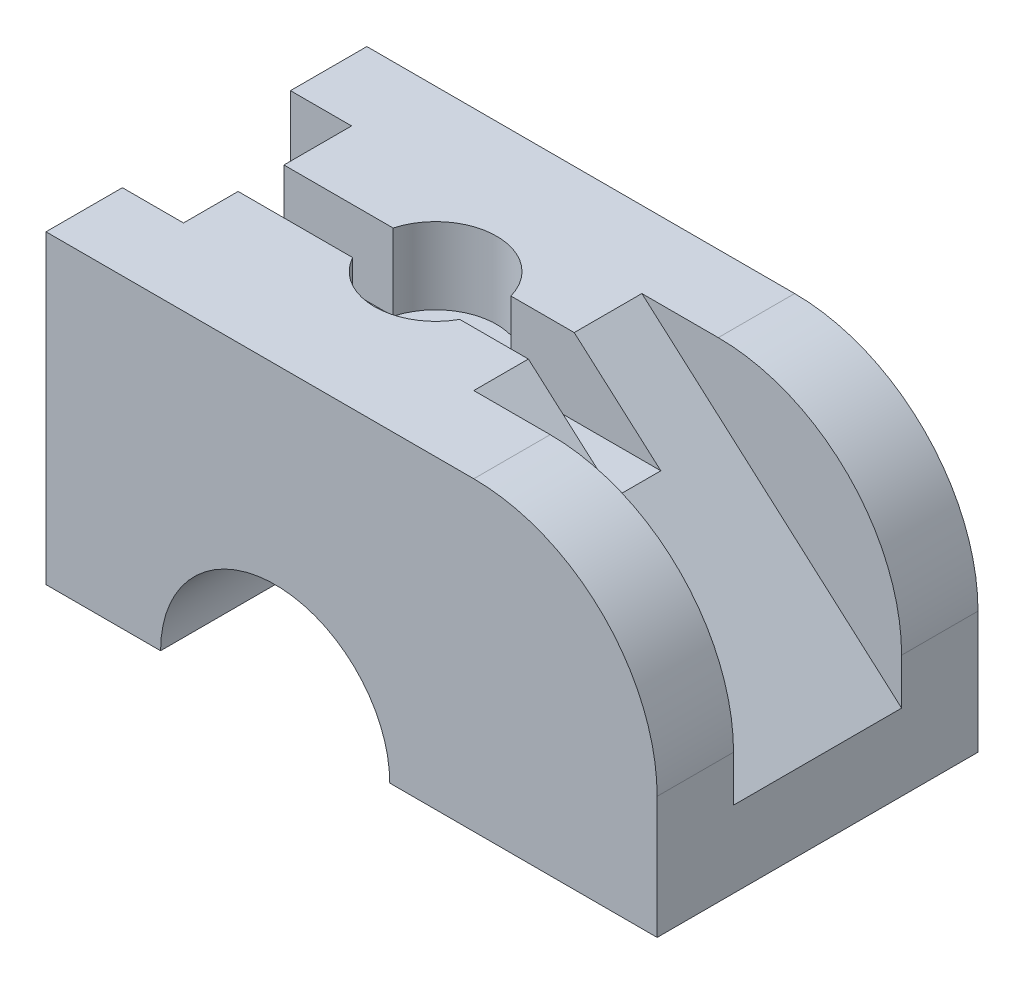
ISO-10303-21;
HEADER;
FILE_DESCRIPTION(('STEP AP214'),'2;1');
FILE_NAME('part.step','',(''),(''),'','','');
FILE_SCHEMA(('AUTOMOTIVE_DESIGN { 1 0 10303 214 1 1 1 1 }'));
ENDSEC;
DATA;
#1=APPLICATION_CONTEXT('core data for automotive mechanical design processes');
#2=APPLICATION_PROTOCOL_DEFINITION('international standard','automotive_design',2000,#1);
#3=PRODUCT_CONTEXT('',#1,'mechanical');
#4=PRODUCT('Part','Part','',(#3));
#5=PRODUCT_RELATED_PRODUCT_CATEGORY('part','',(#4));
#6=PRODUCT_DEFINITION_FORMATION('','',#4);
#7=PRODUCT_DEFINITION_CONTEXT('part definition',#1,'design');
#8=PRODUCT_DEFINITION('design','',#6,#7);
#9=PRODUCT_DEFINITION_SHAPE('','',#8);
#10=(LENGTH_UNIT() NAMED_UNIT(*) SI_UNIT(.MILLI.,.METRE.));
#11=(NAMED_UNIT(*) PLANE_ANGLE_UNIT() SI_UNIT($,.RADIAN.));
#12=(NAMED_UNIT(*) SI_UNIT($,.STERADIAN.) SOLID_ANGLE_UNIT());
#13=UNCERTAINTY_MEASURE_WITH_UNIT(LENGTH_MEASURE(1.E-05),#10,'distance_accuracy_value','');
#14=(GEOMETRIC_REPRESENTATION_CONTEXT(3) GLOBAL_UNCERTAINTY_ASSIGNED_CONTEXT((#13)) GLOBAL_UNIT_ASSIGNED_CONTEXT((#10,
#11,#12)) REPRESENTATION_CONTEXT('',''));
#15=CARTESIAN_POINT('',(0.,0.,0.));
#16=DIRECTION('',(0.,0.,1.));
#17=DIRECTION('',(1.,0.,0.));
#18=AXIS2_PLACEMENT_3D('',#15,#16,#17);
#19=CARTESIAN_POINT('',(-40.,0.,-42.));
#20=DIRECTION('',(-1.,0.,0.));
#21=DIRECTION('',(0.,0.,1.));
#22=AXIS2_PLACEMENT_3D('',#19,#20,#21);
#23=PLANE('',#22);
#24=DIRECTION('',(0.,1.,0.));
#25=VECTOR('',#24,1.);
#26=CARTESIAN_POINT('',(-40.,-2.,-32.));
#27=LINE('',#26,#25);
#28=CARTESIAN_POINT('',(-40.,0.,-32.));
#29=VERTEX_POINT('',#28);
#30=CARTESIAN_POINT('',(-40.,40.,-32.));
#31=VERTEX_POINT('',#30);
#32=EDGE_CURVE('E392',#29,#31,#27,.T.);
#33=ORIENTED_EDGE('',*,*,#32,.T.);
#34=DIRECTION('',(0.,0.,1.));
#35=VECTOR('',#34,1.);
#36=CARTESIAN_POINT('',(-40.,40.,-42.));
#37=LINE('',#36,#35);
#38=CARTESIAN_POINT('',(-40.,40.,-42.));
#39=VERTEX_POINT('',#38);
#40=EDGE_CURVE('E226',#39,#31,#37,.T.);
#41=ORIENTED_EDGE('',*,*,#40,.F.);
#42=DIRECTION('',(0.,-1.,0.));
#43=VECTOR('',#42,1.);
#44=CARTESIAN_POINT('',(-40.,0.,-42.));
#45=LINE('',#44,#43);
#46=CARTESIAN_POINT('',(-40.,0.,-42.));
#47=VERTEX_POINT('',#46);
#48=EDGE_CURVE('E335',#39,#47,#45,.T.);
#49=ORIENTED_EDGE('',*,*,#48,.T.);
#50=DIRECTION('',(0.,0.,1.));
#51=VECTOR('',#50,1.);
#52=CARTESIAN_POINT('',(-40.,0.,-42.));
#53=LINE('',#52,#51);
#54=EDGE_CURVE('E238',#47,#29,#53,.T.);
#55=ORIENTED_EDGE('',*,*,#54,.T.);
#56=EDGE_LOOP('',(#33,#41,#49,#55));
#57=FACE_BOUND('',#56,.T.);
#58=ADVANCED_FACE('F50',(#57),#23,.T.);
#59=CARTESIAN_POINT('',(-40.,0.,-42.));
#60=DIRECTION('',(0.,-1.,0.));
#61=DIRECTION('',(0.,0.,-1.));
#62=AXIS2_PLACEMENT_3D('',#59,#60,#61);
#63=PLANE('',#62);
#64=DIRECTION('',(0.,0.,1.));
#65=VECTOR('',#64,1.);
#66=CARTESIAN_POINT('',(5.,0.,-42.));
#67=LINE('',#66,#65);
#68=CARTESIAN_POINT('',(5.,0.,-42.));
#69=VERTEX_POINT('',#68);
#70=CARTESIAN_POINT('',(5.,0.,0.));
#71=VERTEX_POINT('',#70);
#72=EDGE_CURVE('E69',#69,#71,#67,.T.);
#73=ORIENTED_EDGE('',*,*,#72,.F.);
#74=DIRECTION('',(1.,0.,0.));
#75=VECTOR('',#74,1.);
#76=CARTESIAN_POINT('',(-40.,0.,-42.));
#77=LINE('',#76,#75);
#78=CARTESIAN_POINT('',(40.,0.,-42.));
#79=VERTEX_POINT('',#78);
#80=EDGE_CURVE('E323',#69,#79,#77,.T.);
#81=ORIENTED_EDGE('',*,*,#80,.T.);
#82=DIRECTION('',(0.,0.,1.));
#83=VECTOR('',#82,1.);
#84=CARTESIAN_POINT('',(40.,0.,-42.));
#85=LINE('',#84,#83);
#86=CARTESIAN_POINT('',(40.,0.,0.));
#87=VERTEX_POINT('',#86);
#88=EDGE_CURVE('E242',#79,#87,#85,.T.);
#89=ORIENTED_EDGE('',*,*,#88,.T.);
#90=DIRECTION('',(1.,0.,0.));
#91=VECTOR('',#90,1.);
#92=CARTESIAN_POINT('',(-40.,0.,0.));
#93=LINE('',#92,#91);
#94=EDGE_CURVE('E295',#71,#87,#93,.T.);
#95=ORIENTED_EDGE('',*,*,#94,.F.);
#96=EDGE_LOOP('',(#73,#81,#89,#95));
#97=FACE_BOUND('',#96,.T.);
#98=ADVANCED_FACE('F321',(#97),#63,.T.);
#99=CARTESIAN_POINT('',(6.,40.,-42.));
#100=DIRECTION('',(-0.661621637086846,-0.749837855365093,0.));
#101=DIRECTION('',(0.749837855365093,-0.661621637086846,0.));
#102=AXIS2_PLACEMENT_3D('',#99,#100,#101);
#103=PLANE('',#102);
#104=DIRECTION('',(0.,0.,1.));
#105=VECTOR('',#104,1.);
#106=CARTESIAN_POINT('',(40.,10.,-42.));
#107=LINE('',#106,#105);
#108=CARTESIAN_POINT('',(40.,10.,-32.));
#109=VERTEX_POINT('',#108);
#110=CARTESIAN_POINT('',(40.,10.,-10.));
#111=VERTEX_POINT('',#110);
#112=EDGE_CURVE('E281',#109,#111,#107,.T.);
#113=ORIENTED_EDGE('',*,*,#112,.F.);
#114=DIRECTION('',(-0.749837855365093,0.661621637086846,0.));
#115=VECTOR('',#114,1.);
#116=CARTESIAN_POINT('',(6.,40.,-32.));
#117=LINE('',#116,#115);
#118=CARTESIAN_POINT('',(6.,40.,-32.));
#119=VERTEX_POINT('',#118);
#120=EDGE_CURVE('E282',#109,#119,#117,.T.);
#121=ORIENTED_EDGE('',*,*,#120,.T.);
#122=DIRECTION('',(0.,0.,1.));
#123=VECTOR('',#122,1.);
#124=CARTESIAN_POINT('',(6.,40.,-42.));
#125=LINE('',#124,#123);
#126=CARTESIAN_POINT('',(6.,40.,-23.147915887961));
#127=VERTEX_POINT('',#126);
#128=EDGE_CURVE('E374',#119,#127,#125,.T.);
#129=ORIENTED_EDGE('',*,*,#128,.T.);
#130=DIRECTION('',(0.749837855365093,-0.661621637086846,0.));
#131=VECTOR('',#130,1.);
#132=CARTESIAN_POINT('',(6.,40.,-23.147915887961));
#133=LINE('',#132,#131);
#134=CARTESIAN_POINT('',(17.3333333333333,30.,-23.147915887961));
#135=VERTEX_POINT('',#134);
#136=EDGE_CURVE('E239',#127,#135,#133,.T.);
#137=ORIENTED_EDGE('',*,*,#136,.T.);
#138=DIRECTION('',(0.,0.,1.));
#139=VECTOR('',#138,1.);
#140=CARTESIAN_POINT('',(17.3333333333333,30.,-42.));
#141=LINE('',#140,#139);
#142=CARTESIAN_POINT('',(17.3333333333333,30.,-17.147915887961));
#143=VERTEX_POINT('',#142);
#144=EDGE_CURVE('E243',#135,#143,#141,.T.);
#145=ORIENTED_EDGE('',*,*,#144,.T.);
#146=DIRECTION('',(-0.749837855365093,0.661621637086846,0.));
#147=VECTOR('',#146,1.);
#148=CARTESIAN_POINT('',(5.99999999999999,40.,-17.147915887961));
#149=LINE('',#148,#147);
#150=CARTESIAN_POINT('',(6.,40.,-17.147915887961));
#151=VERTEX_POINT('',#150);
#152=EDGE_CURVE('E250',#143,#151,#149,.T.);
#153=ORIENTED_EDGE('',*,*,#152,.T.);
#154=CARTESIAN_POINT('',(6.,40.,-10.));
#155=VERTEX_POINT('',#154);
#156=EDGE_CURVE('E380',#151,#155,#125,.T.);
#157=ORIENTED_EDGE('',*,*,#156,.T.);
#158=DIRECTION('',(-0.749837855365093,0.661621637086846,0.));
#159=VECTOR('',#158,1.);
#160=CARTESIAN_POINT('',(6.,40.,-10.));
#161=LINE('',#160,#159);
#162=EDGE_CURVE('E248',#111,#155,#161,.T.);
#163=ORIENTED_EDGE('',*,*,#162,.F.);
#164=EDGE_LOOP('',(#113,#121,#129,#137,#145,#153,#157,#163));
#165=FACE_BOUND('',#164,.T.);
#166=ADVANCED_FACE('F430',(#165),#103,.F.);
#167=CARTESIAN_POINT('',(-40.,40.,-42.));
#168=DIRECTION('',(0.,1.,0.));
#169=DIRECTION('',(0.,0.,1.));
#170=AXIS2_PLACEMENT_3D('',#167,#168,#169);
#171=PLANE('',#170);
#172=DIRECTION('',(-1.,0.,0.));
#173=VECTOR('',#172,1.);
#174=CARTESIAN_POINT('',(-40.,40.,-32.));
#175=LINE('',#174,#173);
#176=CARTESIAN_POINT('',(-32.,40.,-32.));
#177=VERTEX_POINT('',#176);
#178=EDGE_CURVE('E215',#177,#31,#175,.T.);
#179=ORIENTED_EDGE('',*,*,#178,.F.);
#180=DIRECTION('',(0.,0.,-1.));
#181=VECTOR('',#180,1.);
#182=CARTESIAN_POINT('',(-32.,40.,-32.));
#183=LINE('',#182,#181);
#184=CARTESIAN_POINT('',(-32.,40.,-23.147915887961));
#185=VERTEX_POINT('',#184);
#186=EDGE_CURVE('E225',#185,#177,#183,.T.);
#187=ORIENTED_EDGE('',*,*,#186,.F.);
#188=DIRECTION('',(-1.,0.,0.));
#189=VECTOR('',#188,1.);
#190=CARTESIAN_POINT('',(-40.,40.,-23.147915887961));
#191=LINE('',#190,#189);
#192=CARTESIAN_POINT('',(-17.7062609181266,40.,-23.147915887961));
#193=VERTEX_POINT('',#192);
#194=EDGE_CURVE('E358',#193,#185,#191,.T.);
#195=ORIENTED_EDGE('',*,*,#194,.F.);
#196=CARTESIAN_POINT('',(-10.,40.,-21.));
#197=DIRECTION('',(0.,1.,0.));
#198=DIRECTION('',(0.,0.,1.));
#199=AXIS2_PLACEMENT_3D('',#196,#197,#198);
#200=CIRCLE('',#199,8.);
#201=CARTESIAN_POINT('',(-2.29373908187345,40.,-23.147915887961));
#202=VERTEX_POINT('',#201);
#203=EDGE_CURVE('E360',#202,#193,#200,.T.);
#204=ORIENTED_EDGE('',*,*,#203,.F.);
#205=DIRECTION('',(-1.,0.,0.));
#206=VECTOR('',#205,1.);
#207=CARTESIAN_POINT('',(-2.29373908187345,40.,-23.147915887961));
#208=LINE('',#207,#206);
#209=EDGE_CURVE('E343',#127,#202,#208,.T.);
#210=ORIENTED_EDGE('',*,*,#209,.F.);
#211=ORIENTED_EDGE('',*,*,#128,.F.);
#212=DIRECTION('',(1.,0.,0.));
#213=VECTOR('',#212,1.);
#214=CARTESIAN_POINT('',(-40.,40.,-32.));
#215=LINE('',#214,#213);
#216=CARTESIAN_POINT('',(16.,40.,-32.));
#217=VERTEX_POINT('',#216);
#218=EDGE_CURVE('E322',#119,#217,#215,.T.);
#219=ORIENTED_EDGE('',*,*,#218,.T.);
#220=DIRECTION('',(0.,0.,-1.));
#221=VECTOR('',#220,1.);
#222=CARTESIAN_POINT('',(16.,40.,-42.));
#223=LINE('',#222,#221);
#224=CARTESIAN_POINT('',(16.,40.,-42.));
#225=VERTEX_POINT('',#224);
#226=EDGE_CURVE('E255',#217,#225,#223,.T.);
#227=ORIENTED_EDGE('',*,*,#226,.T.);
#228=DIRECTION('',(-1.,0.,0.));
#229=VECTOR('',#228,1.);
#230=CARTESIAN_POINT('',(6.,40.,-42.));
#231=LINE('',#230,#229);
#232=EDGE_CURVE('E305',#225,#39,#231,.T.);
#233=ORIENTED_EDGE('',*,*,#232,.T.);
#234=ORIENTED_EDGE('',*,*,#40,.T.);
#235=EDGE_LOOP('',(#179,#187,#195,#204,#210,#211,#219,#227,#233,#234));
#236=FACE_BOUND('',#235,.T.);
#237=ADVANCED_FACE('F407',(#236),#171,.T.);
#238=CARTESIAN_POINT('',(40.,15.9999999999998,-42.));
#239=DIRECTION('',(1.,0.,0.));
#240=DIRECTION('',(0.,0.,-1.));
#241=AXIS2_PLACEMENT_3D('',#238,#239,#240);
#242=PLANE('',#241);
#243=DIRECTION('',(0.,1.,0.));
#244=VECTOR('',#243,1.);
#245=CARTESIAN_POINT('',(40.,0.,-42.));
#246=LINE('',#245,#244);
#247=CARTESIAN_POINT('',(40.,16.,-42.));
#248=VERTEX_POINT('',#247);
#249=EDGE_CURVE('E230',#79,#248,#246,.T.);
#250=ORIENTED_EDGE('',*,*,#249,.T.);
#251=DIRECTION('',(0.,0.,-1.));
#252=VECTOR('',#251,1.);
#253=CARTESIAN_POINT('',(40.,16.,-42.));
#254=LINE('',#253,#252);
#255=CARTESIAN_POINT('',(40.,16.,-32.));
#256=VERTEX_POINT('',#255);
#257=EDGE_CURVE('E257',#248,#256,#254,.F.);
#258=ORIENTED_EDGE('',*,*,#257,.T.);
#259=DIRECTION('',(0.,-1.,0.));
#260=VECTOR('',#259,1.);
#261=CARTESIAN_POINT('',(40.,40.,-32.));
#262=LINE('',#261,#260);
#263=EDGE_CURVE('E385',#256,#109,#262,.T.);
#264=ORIENTED_EDGE('',*,*,#263,.T.);
#265=ORIENTED_EDGE('',*,*,#112,.T.);
#266=DIRECTION('',(0.,1.,0.));
#267=VECTOR('',#266,1.);
#268=CARTESIAN_POINT('',(40.,40.,-10.));
#269=LINE('',#268,#267);
#270=CARTESIAN_POINT('',(40.,16.,-10.));
#271=VERTEX_POINT('',#270);
#272=EDGE_CURVE('E271',#111,#271,#269,.T.);
#273=ORIENTED_EDGE('',*,*,#272,.T.);
#274=DIRECTION('',(0.,0.,1.));
#275=VECTOR('',#274,1.);
#276=CARTESIAN_POINT('',(40.,16.,-42.));
#277=LINE('',#276,#275);
#278=CARTESIAN_POINT('',(40.,16.,0.));
#279=VERTEX_POINT('',#278);
#280=EDGE_CURVE('E256',#271,#279,#277,.T.);
#281=ORIENTED_EDGE('',*,*,#280,.T.);
#282=DIRECTION('',(0.,1.,0.));
#283=VECTOR('',#282,1.);
#284=CARTESIAN_POINT('',(40.,15.9999999999998,0.));
#285=LINE('',#284,#283);
#286=EDGE_CURVE('E293',#87,#279,#285,.T.);
#287=ORIENTED_EDGE('',*,*,#286,.F.);
#288=ORIENTED_EDGE('',*,*,#88,.F.);
#289=EDGE_LOOP('',(#250,#258,#264,#265,#273,#281,#287,#288));
#290=FACE_BOUND('',#289,.T.);
#291=ADVANCED_FACE('F278',(#290),#242,.T.);
#292=DIRECTION('',(1.,0.,0.));
#293=VECTOR('',#292,1.);
#294=CARTESIAN_POINT('',(-40.,0.,-32.));
#295=LINE('',#294,#293);
#296=CARTESIAN_POINT('',(-32.,0.,-32.));
#297=VERTEX_POINT('',#296);
#298=EDGE_CURVE('E318',#29,#297,#295,.T.);
#299=ORIENTED_EDGE('',*,*,#298,.F.);
#300=ORIENTED_EDGE('',*,*,#54,.F.);
#301=CARTESIAN_POINT('',(-25.,0.,-42.));
#302=VERTEX_POINT('',#301);
#303=EDGE_CURVE('E234',#47,#302,#77,.T.);
#304=ORIENTED_EDGE('',*,*,#303,.T.);
#305=DIRECTION('',(0.,0.,1.));
#306=VECTOR('',#305,1.);
#307=CARTESIAN_POINT('',(-25.,0.,-42.));
#308=LINE('',#307,#306);
#309=CARTESIAN_POINT('',(-25.,0.,0.));
#310=VERTEX_POINT('',#309);
#311=EDGE_CURVE('E320',#302,#310,#308,.T.);
#312=ORIENTED_EDGE('',*,*,#311,.T.);
#313=CARTESIAN_POINT('',(-40.,0.,0.));
#314=VERTEX_POINT('',#313);
#315=EDGE_CURVE('E297',#314,#310,#93,.T.);
#316=ORIENTED_EDGE('',*,*,#315,.F.);
#317=CARTESIAN_POINT('',(-40.,0.,-10.));
#318=VERTEX_POINT('',#317);
#319=EDGE_CURVE('E235',#318,#314,#53,.T.);
#320=ORIENTED_EDGE('',*,*,#319,.F.);
#321=DIRECTION('',(-1.,0.,0.));
#322=VECTOR('',#321,1.);
#323=CARTESIAN_POINT('',(-40.,0.,-10.));
#324=LINE('',#323,#322);
#325=CARTESIAN_POINT('',(-32.,0.,-10.));
#326=VERTEX_POINT('',#325);
#327=EDGE_CURVE('E206',#326,#318,#324,.T.);
#328=ORIENTED_EDGE('',*,*,#327,.F.);
#329=DIRECTION('',(0.,0.,1.));
#330=VECTOR('',#329,1.);
#331=CARTESIAN_POINT('',(-32.,0.,-42.));
#332=LINE('',#331,#330);
#333=EDGE_CURVE('E387',#297,#326,#332,.T.);
#334=ORIENTED_EDGE('',*,*,#333,.F.);
#335=EDGE_LOOP('',(#299,#300,#304,#312,#316,#320,#328,#334));
#336=FACE_BOUND('',#335,.T.);
#337=ADVANCED_FACE('F314',(#336),#63,.T.);
#338=DIRECTION('',(0.,1.,0.));
#339=VECTOR('',#338,1.);
#340=CARTESIAN_POINT('',(-40.,-2.,-10.));
#341=LINE('',#340,#339);
#342=CARTESIAN_POINT('',(-40.,40.,-10.));
#343=VERTEX_POINT('',#342);
#344=EDGE_CURVE('E201',#318,#343,#341,.T.);
#345=ORIENTED_EDGE('',*,*,#344,.F.);
#346=ORIENTED_EDGE('',*,*,#319,.T.);
#347=DIRECTION('',(0.,-1.,0.));
#348=VECTOR('',#347,1.);
#349=CARTESIAN_POINT('',(-40.,0.,0.));
#350=LINE('',#349,#348);
#351=CARTESIAN_POINT('',(-40.,40.,0.));
#352=VERTEX_POINT('',#351);
#353=EDGE_CURVE('E227',#352,#314,#350,.T.);
#354=ORIENTED_EDGE('',*,*,#353,.F.);
#355=EDGE_CURVE('E216',#343,#352,#37,.T.);
#356=ORIENTED_EDGE('',*,*,#355,.F.);
#357=EDGE_LOOP('',(#345,#346,#354,#356));
#358=FACE_BOUND('',#357,.T.);
#359=ADVANCED_FACE('F224',(#358),#23,.T.);
#360=CARTESIAN_POINT('',(-32.,40.,-10.));
#361=VERTEX_POINT('',#360);
#362=CARTESIAN_POINT('',(-32.,40.,-17.147915887961));
#363=VERTEX_POINT('',#362);
#364=EDGE_CURVE('E221',#361,#363,#183,.T.);
#365=ORIENTED_EDGE('',*,*,#364,.F.);
#366=DIRECTION('',(1.,0.,0.));
#367=VECTOR('',#366,1.);
#368=CARTESIAN_POINT('',(-32.,40.,-10.));
#369=LINE('',#368,#367);
#370=EDGE_CURVE('E204',#343,#361,#369,.T.);
#371=ORIENTED_EDGE('',*,*,#370,.F.);
#372=ORIENTED_EDGE('',*,*,#355,.T.);
#373=DIRECTION('',(-1.,0.,0.));
#374=VECTOR('',#373,1.);
#375=CARTESIAN_POINT('',(-40.,40.,0.));
#376=LINE('',#375,#374);
#377=CARTESIAN_POINT('',(16.,40.,0.));
#378=VERTEX_POINT('',#377);
#379=EDGE_CURVE('E289',#378,#352,#376,.T.);
#380=ORIENTED_EDGE('',*,*,#379,.F.);
#381=DIRECTION('',(0.,0.,1.));
#382=VECTOR('',#381,1.);
#383=CARTESIAN_POINT('',(16.,40.,-42.));
#384=LINE('',#383,#382);
#385=CARTESIAN_POINT('',(16.,40.,-10.));
#386=VERTEX_POINT('',#385);
#387=EDGE_CURVE('E266',#378,#386,#384,.F.);
#388=ORIENTED_EDGE('',*,*,#387,.T.);
#389=DIRECTION('',(-1.,0.,0.));
#390=VECTOR('',#389,1.);
#391=CARTESIAN_POINT('',(-40.,40.,-10.));
#392=LINE('',#391,#390);
#393=EDGE_CURVE('E274',#386,#155,#392,.T.);
#394=ORIENTED_EDGE('',*,*,#393,.T.);
#395=ORIENTED_EDGE('',*,*,#156,.F.);
#396=DIRECTION('',(1.,0.,0.));
#397=VECTOR('',#396,1.);
#398=CARTESIAN_POINT('',(6.,40.,-17.147915887961));
#399=LINE('',#398,#397);
#400=CARTESIAN_POINT('',(-2.98847748390004,40.,-17.147915887961));
#401=VERTEX_POINT('',#400);
#402=EDGE_CURVE('E346',#401,#151,#399,.T.);
#403=ORIENTED_EDGE('',*,*,#402,.F.);
#404=CARTESIAN_POINT('',(-10.,40.,-21.));
#405=DIRECTION('',(0.,1.,0.));
#406=DIRECTION('',(0.,0.,1.));
#407=AXIS2_PLACEMENT_3D('',#404,#405,#406);
#408=CIRCLE('',#407,8.);
#409=CARTESIAN_POINT('',(-17.0115225161,40.,-17.147915887961));
#410=VERTEX_POINT('',#409);
#411=EDGE_CURVE('E351',#410,#401,#408,.T.);
#412=ORIENTED_EDGE('',*,*,#411,.F.);
#413=DIRECTION('',(1.,0.,0.));
#414=VECTOR('',#413,1.);
#415=CARTESIAN_POINT('',(-17.0115225161,40.,-17.147915887961));
#416=LINE('',#415,#414);
#417=EDGE_CURVE('E353',#363,#410,#416,.T.);
#418=ORIENTED_EDGE('',*,*,#417,.F.);
#419=EDGE_LOOP('',(#365,#371,#372,#380,#388,#394,#395,#403,#412,#418));
#420=FACE_BOUND('',#419,.T.);
#421=ADVANCED_FACE('F218',(#420),#171,.T.);
#422=CARTESIAN_POINT('',(16.,16.,-42.));
#423=DIRECTION('',(0.,0.,-1.));
#424=DIRECTION('',(-1.,0.,0.));
#425=AXIS2_PLACEMENT_3D('',#422,#423,#424);
#426=PLANE('',#425);
#427=CARTESIAN_POINT('',(-10.,0.,-42.));
#428=DIRECTION('',(0.,0.,1.));
#429=DIRECTION('',(1.,0.,0.));
#430=AXIS2_PLACEMENT_3D('',#427,#428,#429);
#431=CIRCLE('',#430,15.);
#432=EDGE_CURVE('E316',#69,#302,#431,.T.);
#433=ORIENTED_EDGE('',*,*,#432,.T.);
#434=ORIENTED_EDGE('',*,*,#303,.F.);
#435=ORIENTED_EDGE('',*,*,#48,.F.);
#436=ORIENTED_EDGE('',*,*,#232,.F.);
#437=CARTESIAN_POINT('',(16.,16.,-42.));
#438=DIRECTION('',(0.,0.,-1.));
#439=DIRECTION('',(-1.,0.,0.));
#440=AXIS2_PLACEMENT_3D('',#437,#438,#439);
#441=CIRCLE('',#440,24.);
#442=EDGE_CURVE('E253',#225,#248,#441,.T.);
#443=ORIENTED_EDGE('',*,*,#442,.T.);
#444=ORIENTED_EDGE('',*,*,#249,.F.);
#445=ORIENTED_EDGE('',*,*,#80,.F.);
#446=EDGE_LOOP('',(#433,#434,#435,#436,#443,#444,#445));
#447=FACE_BOUND('',#446,.T.);
#448=ADVANCED_FACE('F327',(#447),#426,.T.);
#449=CARTESIAN_POINT('',(16.,16.,0.));
#450=DIRECTION('',(0.,0.,-1.));
#451=DIRECTION('',(-1.,0.,0.));
#452=AXIS2_PLACEMENT_3D('',#449,#450,#451);
#453=PLANE('',#452);
#454=ORIENTED_EDGE('',*,*,#315,.T.);
#455=CARTESIAN_POINT('',(-10.,0.,0.));
#456=DIRECTION('',(0.,0.,1.));
#457=DIRECTION('',(1.,0.,0.));
#458=AXIS2_PLACEMENT_3D('',#455,#456,#457);
#459=CIRCLE('',#458,15.);
#460=EDGE_CURVE('E319',#71,#310,#459,.T.);
#461=ORIENTED_EDGE('',*,*,#460,.F.);
#462=ORIENTED_EDGE('',*,*,#94,.T.);
#463=ORIENTED_EDGE('',*,*,#286,.T.);
#464=CARTESIAN_POINT('',(16.,16.,0.));
#465=DIRECTION('',(0.,0.,-1.));
#466=DIRECTION('',(-1.,0.,0.));
#467=AXIS2_PLACEMENT_3D('',#464,#465,#466);
#468=CIRCLE('',#467,24.);
#469=EDGE_CURVE('E264',#279,#378,#468,.F.);
#470=ORIENTED_EDGE('',*,*,#469,.T.);
#471=ORIENTED_EDGE('',*,*,#379,.T.);
#472=ORIENTED_EDGE('',*,*,#353,.T.);
#473=EDGE_LOOP('',(#454,#461,#462,#463,#470,#471,#472));
#474=FACE_BOUND('',#473,.T.);
#475=ADVANCED_FACE('F288',(#474),#453,.F.);
#476=CARTESIAN_POINT('',(-10.,30.,-21.));
#477=DIRECTION('',(0.,1.,0.));
#478=DIRECTION('',(0.,0.,1.));
#479=AXIS2_PLACEMENT_3D('',#476,#477,#478);
#480=CYLINDRICAL_SURFACE('',#479,8.);
#481=ORIENTED_EDGE('',*,*,#203,.T.);
#482=DIRECTION('',(0.,1.,0.));
#483=VECTOR('',#482,1.);
#484=CARTESIAN_POINT('',(-17.7062609181266,30.,-23.147915887961));
#485=LINE('',#484,#483);
#486=CARTESIAN_POINT('',(-17.7062609181266,30.,-23.147915887961));
#487=VERTEX_POINT('',#486);
#488=EDGE_CURVE('E337',#487,#193,#485,.T.);
#489=ORIENTED_EDGE('',*,*,#488,.F.);
#490=CARTESIAN_POINT('',(-10.,30.,-21.));
#491=DIRECTION('',(0.,1.,0.));
#492=DIRECTION('',(0.,0.,1.));
#493=AXIS2_PLACEMENT_3D('',#490,#491,#492);
#494=CIRCLE('',#493,8.);
#495=CARTESIAN_POINT('',(-2.29373908187345,30.,-23.147915887961));
#496=VERTEX_POINT('',#495);
#497=EDGE_CURVE('E350',#496,#487,#494,.T.);
#498=ORIENTED_EDGE('',*,*,#497,.F.);
#499=DIRECTION('',(0.,1.,0.));
#500=VECTOR('',#499,1.);
#501=CARTESIAN_POINT('',(-2.29373908187345,30.,-23.147915887961));
#502=LINE('',#501,#500);
#503=EDGE_CURVE('E292',#496,#202,#502,.T.);
#504=ORIENTED_EDGE('',*,*,#503,.T.);
#505=EDGE_LOOP('',(#481,#489,#498,#504));
#506=FACE_BOUND('',#505,.T.);
#507=ADVANCED_FACE('F454',(#506),#480,.F.);
#508=CARTESIAN_POINT('',(-2.29373908187345,30.,-23.147915887961));
#509=DIRECTION('',(0.,0.,-1.));
#510=DIRECTION('',(-1.,0.,0.));
#511=AXIS2_PLACEMENT_3D('',#508,#509,#510);
#512=PLANE('',#511);
#513=ORIENTED_EDGE('',*,*,#209,.T.);
#514=ORIENTED_EDGE('',*,*,#503,.F.);
#515=DIRECTION('',(-1.,0.,0.));
#516=VECTOR('',#515,1.);
#517=CARTESIAN_POINT('',(-2.29373908187345,30.,-23.147915887961));
#518=LINE('',#517,#516);
#519=EDGE_CURVE('E338',#135,#496,#518,.T.);
#520=ORIENTED_EDGE('',*,*,#519,.F.);
#521=ORIENTED_EDGE('',*,*,#136,.F.);
#522=EDGE_LOOP('',(#513,#514,#520,#521));
#523=FACE_BOUND('',#522,.T.);
#524=ADVANCED_FACE('F452',(#523),#512,.F.);
#525=CARTESIAN_POINT('',(6.,30.,-17.147915887961));
#526=DIRECTION('',(0.,0.,1.));
#527=DIRECTION('',(1.,0.,0.));
#528=AXIS2_PLACEMENT_3D('',#525,#526,#527);
#529=PLANE('',#528);
#530=ORIENTED_EDGE('',*,*,#402,.T.);
#531=ORIENTED_EDGE('',*,*,#152,.F.);
#532=DIRECTION('',(1.,0.,0.));
#533=VECTOR('',#532,1.);
#534=CARTESIAN_POINT('',(6.,30.,-17.147915887961));
#535=LINE('',#534,#533);
#536=CARTESIAN_POINT('',(-2.98847748390004,30.,-17.147915887961));
#537=VERTEX_POINT('',#536);
#538=EDGE_CURVE('E361',#537,#143,#535,.T.);
#539=ORIENTED_EDGE('',*,*,#538,.F.);
#540=DIRECTION('',(0.,1.,0.));
#541=VECTOR('',#540,1.);
#542=CARTESIAN_POINT('',(-2.98847748390004,30.,-17.147915887961));
#543=LINE('',#542,#541);
#544=EDGE_CURVE('E298',#537,#401,#543,.T.);
#545=ORIENTED_EDGE('',*,*,#544,.T.);
#546=EDGE_LOOP('',(#530,#531,#539,#545));
#547=FACE_BOUND('',#546,.T.);
#548=ADVANCED_FACE('F432',(#547),#529,.F.);
#549=CARTESIAN_POINT('',(-10.,30.,-21.));
#550=DIRECTION('',(0.,1.,0.));
#551=DIRECTION('',(0.,0.,1.));
#552=AXIS2_PLACEMENT_3D('',#549,#550,#551);
#553=CYLINDRICAL_SURFACE('',#552,8.);
#554=ORIENTED_EDGE('',*,*,#411,.T.);
#555=ORIENTED_EDGE('',*,*,#544,.F.);
#556=CARTESIAN_POINT('',(-10.,30.,-21.));
#557=DIRECTION('',(0.,1.,0.));
#558=DIRECTION('',(0.,0.,1.));
#559=AXIS2_PLACEMENT_3D('',#556,#557,#558);
#560=CIRCLE('',#559,8.);
#561=CARTESIAN_POINT('',(-17.0115225161,30.,-17.147915887961));
#562=VERTEX_POINT('',#561);
#563=EDGE_CURVE('E362',#562,#537,#560,.T.);
#564=ORIENTED_EDGE('',*,*,#563,.F.);
#565=DIRECTION('',(0.,1.,0.));
#566=VECTOR('',#565,1.);
#567=CARTESIAN_POINT('',(-17.0115225161,30.,-17.147915887961));
#568=LINE('',#567,#566);
#569=EDGE_CURVE('E339',#562,#410,#568,.T.);
#570=ORIENTED_EDGE('',*,*,#569,.T.);
#571=EDGE_LOOP('',(#554,#555,#564,#570));
#572=FACE_BOUND('',#571,.T.);
#573=ADVANCED_FACE('F438',(#572),#553,.F.);
#574=CARTESIAN_POINT('',(-17.0115225161,30.,-17.147915887961));
#575=DIRECTION('',(0.,0.,1.));
#576=DIRECTION('',(1.,0.,0.));
#577=AXIS2_PLACEMENT_3D('',#574,#575,#576);
#578=PLANE('',#577);
#579=DIRECTION('',(1.,0.,0.));
#580=VECTOR('',#579,1.);
#581=CARTESIAN_POINT('',(-17.0115225161,30.,-17.147915887961));
#582=LINE('',#581,#580);
#583=CARTESIAN_POINT('',(-32.,30.,-17.147915887961));
#584=VERTEX_POINT('',#583);
#585=EDGE_CURVE('E368',#584,#562,#582,.T.);
#586=ORIENTED_EDGE('',*,*,#585,.F.);
#587=DIRECTION('',(0.,1.,0.));
#588=VECTOR('',#587,1.);
#589=CARTESIAN_POINT('',(-32.,30.,-17.147915887961));
#590=LINE('',#589,#588);
#591=EDGE_CURVE('E64',#584,#363,#590,.T.);
#592=ORIENTED_EDGE('',*,*,#591,.T.);
#593=ORIENTED_EDGE('',*,*,#417,.T.);
#594=ORIENTED_EDGE('',*,*,#569,.F.);
#595=EDGE_LOOP('',(#586,#592,#593,#594));
#596=FACE_BOUND('',#595,.T.);
#597=ADVANCED_FACE('F445',(#596),#578,.F.);
#598=CARTESIAN_POINT('',(-40.,30.,-23.147915887961));
#599=DIRECTION('',(0.,0.,-1.));
#600=DIRECTION('',(-1.,0.,0.));
#601=AXIS2_PLACEMENT_3D('',#598,#599,#600);
#602=PLANE('',#601);
#603=ORIENTED_EDGE('',*,*,#194,.T.);
#604=DIRECTION('',(0.,-1.,0.));
#605=VECTOR('',#604,1.);
#606=CARTESIAN_POINT('',(-32.,30.,-23.147915887961));
#607=LINE('',#606,#605);
#608=CARTESIAN_POINT('',(-32.,30.,-23.147915887961));
#609=VERTEX_POINT('',#608);
#610=EDGE_CURVE('E391',#185,#609,#607,.T.);
#611=ORIENTED_EDGE('',*,*,#610,.T.);
#612=DIRECTION('',(-1.,0.,0.));
#613=VECTOR('',#612,1.);
#614=CARTESIAN_POINT('',(-40.,30.,-23.147915887961));
#615=LINE('',#614,#613);
#616=EDGE_CURVE('E369',#487,#609,#615,.T.);
#617=ORIENTED_EDGE('',*,*,#616,.F.);
#618=ORIENTED_EDGE('',*,*,#488,.T.);
#619=EDGE_LOOP('',(#603,#611,#617,#618));
#620=FACE_BOUND('',#619,.T.);
#621=ADVANCED_FACE('F450',(#620),#602,.F.);
#622=CARTESIAN_POINT('',(-10.,30.,-21.));
#623=DIRECTION('',(0.,1.,0.));
#624=DIRECTION('',(0.,0.,1.));
#625=AXIS2_PLACEMENT_3D('',#622,#623,#624);
#626=PLANE('',#625);
#627=DIRECTION('',(0.,0.,-1.));
#628=VECTOR('',#627,1.);
#629=CARTESIAN_POINT('',(-32.,30.,-21.));
#630=LINE('',#629,#628);
#631=EDGE_CURVE('E11',#584,#609,#630,.T.);
#632=ORIENTED_EDGE('',*,*,#631,.F.);
#633=ORIENTED_EDGE('',*,*,#585,.T.);
#634=ORIENTED_EDGE('',*,*,#563,.T.);
#635=ORIENTED_EDGE('',*,*,#538,.T.);
#636=ORIENTED_EDGE('',*,*,#144,.F.);
#637=ORIENTED_EDGE('',*,*,#519,.T.);
#638=ORIENTED_EDGE('',*,*,#497,.T.);
#639=ORIENTED_EDGE('',*,*,#616,.T.);
#640=EDGE_LOOP('',(#632,#633,#634,#635,#636,#637,#638,#639));
#641=FACE_BOUND('',#640,.T.);
#642=ADVANCED_FACE('F443',(#641),#626,.T.);
#643=CARTESIAN_POINT('',(0.,0.,-10.));
#644=DIRECTION('',(0.,0.,1.));
#645=DIRECTION('',(1.,0.,0.));
#646=AXIS2_PLACEMENT_3D('',#643,#644,#645);
#647=PLANE('',#646);
#648=ORIENTED_EDGE('',*,*,#393,.F.);
#649=CARTESIAN_POINT('',(16.,16.,-10.));
#650=DIRECTION('',(0.,0.,1.));
#651=DIRECTION('',(1.,0.,0.));
#652=AXIS2_PLACEMENT_3D('',#649,#650,#651);
#653=CIRCLE('',#652,24.);
#654=EDGE_CURVE('E54',#386,#271,#653,.F.);
#655=ORIENTED_EDGE('',*,*,#654,.T.);
#656=ORIENTED_EDGE('',*,*,#272,.F.);
#657=ORIENTED_EDGE('',*,*,#162,.T.);
#658=EDGE_LOOP('',(#648,#655,#656,#657));
#659=FACE_BOUND('',#658,.T.);
#660=ADVANCED_FACE('F275',(#659),#647,.F.);
#661=CARTESIAN_POINT('',(0.,0.,-32.));
#662=DIRECTION('',(0.,0.,1.));
#663=DIRECTION('',(1.,0.,0.));
#664=AXIS2_PLACEMENT_3D('',#661,#662,#663);
#665=PLANE('',#664);
#666=ORIENTED_EDGE('',*,*,#263,.F.);
#667=CARTESIAN_POINT('',(16.,16.,-32.));
#668=DIRECTION('',(0.,0.,1.));
#669=DIRECTION('',(1.,0.,0.));
#670=AXIS2_PLACEMENT_3D('',#667,#668,#669);
#671=CIRCLE('',#670,24.);
#672=EDGE_CURVE('E265',#256,#217,#671,.T.);
#673=ORIENTED_EDGE('',*,*,#672,.T.);
#674=ORIENTED_EDGE('',*,*,#218,.F.);
#675=ORIENTED_EDGE('',*,*,#120,.F.);
#676=EDGE_LOOP('',(#666,#673,#674,#675));
#677=FACE_BOUND('',#676,.T.);
#678=ADVANCED_FACE('F424',(#677),#665,.T.);
#679=CARTESIAN_POINT('',(16.,16.,-42.));
#680=DIRECTION('',(0.,0.,-1.));
#681=DIRECTION('',(-1.,0.,0.));
#682=AXIS2_PLACEMENT_3D('',#679,#680,#681);
#683=CYLINDRICAL_SURFACE('',#682,24.);
#684=ORIENTED_EDGE('',*,*,#672,.F.);
#685=ORIENTED_EDGE('',*,*,#257,.F.);
#686=ORIENTED_EDGE('',*,*,#442,.F.);
#687=ORIENTED_EDGE('',*,*,#226,.F.);
#688=EDGE_LOOP('',(#684,#685,#686,#687));
#689=FACE_BOUND('',#688,.T.);
#690=ADVANCED_FACE('F419',(#689),#683,.T.);
#691=CARTESIAN_POINT('',(16.,16.,-42.));
#692=DIRECTION('',(0.,0.,1.));
#693=DIRECTION('',(1.,0.,0.));
#694=AXIS2_PLACEMENT_3D('',#691,#692,#693);
#695=CYLINDRICAL_SURFACE('',#694,24.);
#696=ORIENTED_EDGE('',*,*,#654,.F.);
#697=ORIENTED_EDGE('',*,*,#387,.F.);
#698=ORIENTED_EDGE('',*,*,#469,.F.);
#699=ORIENTED_EDGE('',*,*,#280,.F.);
#700=EDGE_LOOP('',(#696,#697,#698,#699));
#701=FACE_BOUND('',#700,.T.);
#702=ADVANCED_FACE('F47',(#701),#695,.T.);
#703=CARTESIAN_POINT('',(-10.,0.,-42.));
#704=DIRECTION('',(0.,0.,1.));
#705=DIRECTION('',(1.,0.,0.));
#706=AXIS2_PLACEMENT_3D('',#703,#704,#705);
#707=CYLINDRICAL_SURFACE('',#706,15.);
#708=ORIENTED_EDGE('',*,*,#460,.T.);
#709=ORIENTED_EDGE('',*,*,#311,.F.);
#710=ORIENTED_EDGE('',*,*,#432,.F.);
#711=ORIENTED_EDGE('',*,*,#72,.T.);
#712=EDGE_LOOP('',(#708,#709,#710,#711));
#713=FACE_BOUND('',#712,.T.);
#714=ADVANCED_FACE('F658',(#713),#707,.F.);
#715=CARTESIAN_POINT('',(-32.,-2.,-32.));
#716=DIRECTION('',(1.,0.,0.));
#717=DIRECTION('',(0.,0.,-1.));
#718=AXIS2_PLACEMENT_3D('',#715,#716,#717);
#719=PLANE('',#718);
#720=ORIENTED_EDGE('',*,*,#333,.T.);
#721=DIRECTION('',(0.,1.,0.));
#722=VECTOR('',#721,1.);
#723=CARTESIAN_POINT('',(-32.,-2.,-10.));
#724=LINE('',#723,#722);
#725=EDGE_CURVE('E211',#326,#361,#724,.T.);
#726=ORIENTED_EDGE('',*,*,#725,.T.);
#727=ORIENTED_EDGE('',*,*,#364,.T.);
#728=ORIENTED_EDGE('',*,*,#591,.F.);
#729=ORIENTED_EDGE('',*,*,#631,.T.);
#730=ORIENTED_EDGE('',*,*,#610,.F.);
#731=ORIENTED_EDGE('',*,*,#186,.T.);
#732=DIRECTION('',(0.,1.,0.));
#733=VECTOR('',#732,1.);
#734=CARTESIAN_POINT('',(-32.,-2.,-32.));
#735=LINE('',#734,#733);
#736=EDGE_CURVE('E397',#297,#177,#735,.T.);
#737=ORIENTED_EDGE('',*,*,#736,.F.);
#738=EDGE_LOOP('',(#720,#726,#727,#728,#729,#730,#731,#737));
#739=FACE_BOUND('',#738,.T.);
#740=ADVANCED_FACE('F409',(#739),#719,.F.);
#741=CARTESIAN_POINT('',(-40.,-2.,-32.));
#742=DIRECTION('',(0.,0.,-1.));
#743=DIRECTION('',(-1.,0.,0.));
#744=AXIS2_PLACEMENT_3D('',#741,#742,#743);
#745=PLANE('',#744);
#746=ORIENTED_EDGE('',*,*,#298,.T.);
#747=ORIENTED_EDGE('',*,*,#736,.T.);
#748=ORIENTED_EDGE('',*,*,#178,.T.);
#749=ORIENTED_EDGE('',*,*,#32,.F.);
#750=EDGE_LOOP('',(#746,#747,#748,#749));
#751=FACE_BOUND('',#750,.T.);
#752=ADVANCED_FACE('F411',(#751),#745,.F.);
#753=CARTESIAN_POINT('',(-32.,-2.,-10.));
#754=DIRECTION('',(0.,0.,1.));
#755=DIRECTION('',(1.,0.,0.));
#756=AXIS2_PLACEMENT_3D('',#753,#754,#755);
#757=PLANE('',#756);
#758=ORIENTED_EDGE('',*,*,#327,.T.);
#759=ORIENTED_EDGE('',*,*,#344,.T.);
#760=ORIENTED_EDGE('',*,*,#370,.T.);
#761=ORIENTED_EDGE('',*,*,#725,.F.);
#762=EDGE_LOOP('',(#758,#759,#760,#761));
#763=FACE_BOUND('',#762,.T.);
#764=ADVANCED_FACE('F202',(#763),#757,.F.);
#765=CLOSED_SHELL('',(#58,#98,#166,#237,#291,#337,#359,#421,#448,#475,#507,#524,#548,#573,#597,
#621,#642,#660,#678,#690,#702,#714,#740,#752,#764));
#766=MANIFOLD_SOLID_BREP('B2',#765);
#767=ADVANCED_BREP_SHAPE_REPRESENTATION('',(#18,#766),#14);
#768=SHAPE_DEFINITION_REPRESENTATION(#9,#767);
ENDSEC;
END-ISO-10303-21;
